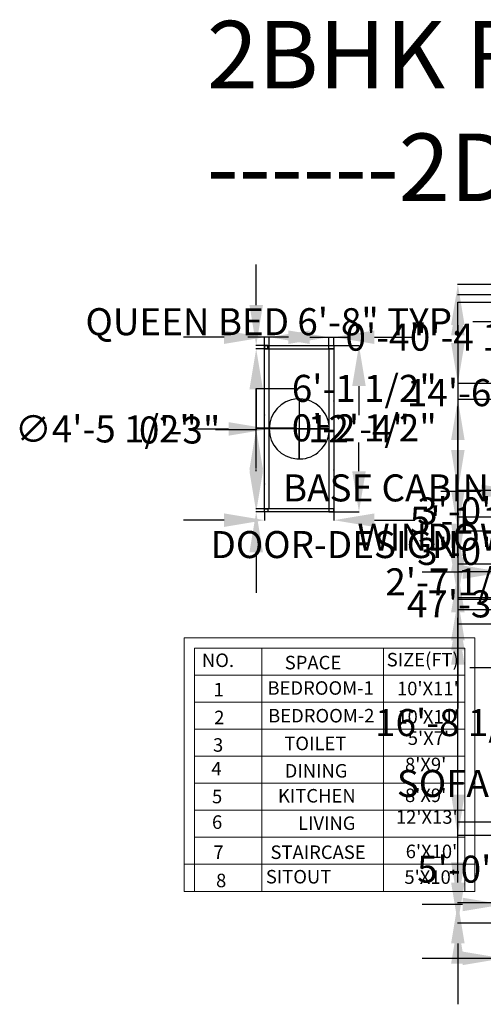
# Model space of a CAD drawing. Units: inches. Extents: x 2838 to 4029, y 1041 to 1915.
# Tile 1 of 16: x 2838 to 3250, y 1041 to 1915. Entities that reach past the tile are written whole.
import ezdxf

# ---------------------------------------------------------------- set-up
doc = ezdxf.new("R2010")
doc.units = ezdxf.units.IN
doc.header["$MEASUREMENT"] = 0
for name, color, linetype, lineweight in [('A-ANNO-DIMS', 2, 'Continuous', 18), ('A-ANNO-SCHD', 7, 'Continuous', 18), ('A-ANNO-TEXT', 7, 'Continuous', 18), ('A-DETL', 7, 'Continuous', 25), ('A-REFR', 8, 'Continuous', 13)]:
    doc.layers.add(name, color=color, linetype=linetype, lineweight=lineweight)
doc.styles.get("Standard").update_dxf_attribs({"font": 'arial.ttf'})
doc.dimstyles.get("Standard").update_dxf_attribs({"dimtxt": 24, "dimasz": 36, "dimexe": 0.18, "dimexo": 0.0625, "dimgap": 0.09, "dimtad": 0, "dimtih": 1, "dimtoh": 1, "dimdec": 0, "dimzin": 0, "dimdsep": 46, "dimlunit": 3, "dimtxsty": 'Standard', "dimcen": 0.09, "dimadec": 0, "dimazin": 0, "dimtfac": 1, "dimtdec": 0, "dimtofl": 0, "dimtmove": 0, "dimatfit": 3, "dimfxl": 1, "dimtolj": 1, "dimtzin": 0, "dimarcsym": 0})

# ---------------------------------------------------------------- blocks, each defined once
blk = doc.blocks.new('*D19')
at = {"layer": 'A-ANNO-DIMS', "color": 0, "lineweight": -2, "transparency": 16777216}
for p, q in [((3117.42, 1626.15), (3139.86, 1626.15)), ((3139.68, 1590.15), (3139.68, 1564.51)), ((3139.68, 1514.59), (3139.68, 1540.23)), ((3117.42, 1478.59), (3139.86, 1478.59))]:
    blk.add_line(p, q, dxfattribs=at)
at = {"layer": 'A-ANNO-DIMS', "color": 0, "transparency": 16777216}
for points in [[(3133.68, 1590.15), (3145.68, 1590.15), (3139.68, 1626.15)], [(3133.68, 1514.59), (3145.68, 1514.59), (3139.68, 1478.59)]]:
    blk.add_solid(points, dxfattribs=at)
at = {"layer": 'Defpoints', "color": 0, "transparency": 16777216}
for p in [(3117.35, 1626.15), (3117.35, 1478.59), (3139.68, 1478.59)]:
    blk.add_point(p, dxfattribs=at)
at = {"layer": 'A-ANNO-DIMS', "color": 0, "transparency": 16777216, "insert": (3139.68, 1552.37), "char_height": 24, "attachment_point": 5}
blk.add_mtext('\\A1;12\'-4"', dxfattribs=at)
blk = doc.blocks.new('*D25')
at = {"layer": 'A-ANNO-DIMS', "color": 0, "lineweight": -2, "transparency": 16777216}
for p, q in [((3283.93, 1516.17), (3283.93, 1552.17)), ((3276.79, 1480.17), (3284.11, 1480.17)), ((3276.79, 1432.17), (3284.11, 1432.17)), ((3283.93, 1396.17), (3283.93, 1360.17))]:
    blk.add_line(p, q, dxfattribs=at)
at = {"layer": 'A-ANNO-DIMS', "color": 0, "transparency": 16777216}
for points in [[(3277.93, 1516.17), (3289.93, 1516.17), (3283.93, 1480.17)], [(3277.93, 1396.17), (3289.93, 1396.17), (3283.93, 1432.17)]]:
    blk.add_solid(points, dxfattribs=at)
at = {"layer": 'Defpoints', "color": 0, "transparency": 16777216}
for p in [(3276.73, 1480.17), (3283.93, 1480.17), (3276.73, 1432.17)]:
    blk.add_point(p, dxfattribs=at)
at = {"layer": 'A-ANNO-DIMS', "color": 0, "transparency": 16777216, "insert": (3283.93, 1456.17), "char_height": 24, "attachment_point": 5}
blk.add_mtext('\\A1;WINDOW 4\'-0" TYP.', dxfattribs=at)
blk = doc.blocks.new('*D26')
at = {"layer": 'A-ANNO-DIMS', "color": 0, "lineweight": -2, "transparency": 16777216}
for p, q in [((3231.73, 1424.97), (3195.73, 1424.97)), ((3267.73, 1432.1), (3267.73, 1424.79)), ((3276.73, 1432.1), (3276.73, 1424.79)), ((3312.73, 1424.97), (3348.73, 1424.97))]:
    blk.add_line(p, q, dxfattribs=at)
at = {"layer": 'A-ANNO-DIMS', "color": 0, "transparency": 16777216}
for points in [[(3231.73, 1430.97), (3231.73, 1418.97), (3267.73, 1424.97)], [(3312.73, 1430.97), (3312.73, 1418.97), (3276.73, 1424.97)]]:
    blk.add_solid(points, dxfattribs=at)
at = {"layer": 'Defpoints', "color": 0, "transparency": 16777216}
for p in [(3267.73, 1432.17), (3276.73, 1432.17), (3276.73, 1424.97)]:
    blk.add_point(p, dxfattribs=at)
at = {"layer": 'A-ANNO-DIMS', "color": 0, "transparency": 16777216, "insert": (3421.97, 1424.97), "char_height": 24, "attachment_point": 5}
blk.add_mtext('\\A1;0\'-9" TYP.', dxfattribs=at)
blk = doc.blocks.new('*D29')
at = {"layer": 'A-ANNO-DIMS', "color": 0, "lineweight": -2, "transparency": 16777216}
for p, q in [((3310.15, 1348.85), (3310.15, 1339.73)), ((3370.15, 1348.85), (3370.15, 1339.73)), ((3274.15, 1339.91), (3238.15, 1339.91)), ((3406.15, 1339.91), (3442.15, 1339.91))]:
    blk.add_line(p, q, dxfattribs=at)
at = {"layer": 'A-ANNO-DIMS', "color": 0, "transparency": 16777216}
for points in [[(3274.15, 1345.91), (3274.15, 1333.91), (3310.15, 1339.91)], [(3406.15, 1345.91), (3406.15, 1333.91), (3370.15, 1339.91)]]:
    blk.add_solid(points, dxfattribs=at)
at = {"layer": 'Defpoints', "color": 0, "transparency": 16777216}
for p in [(3310.15, 1348.91), (3370.15, 1348.91), (3370.15, 1339.91)]:
    blk.add_point(p, dxfattribs=at)
at = {"layer": 'A-ANNO-DIMS', "color": 0, "transparency": 16777216, "insert": (3566.77, 1339.91), "char_height": 24, "attachment_point": 5}
blk.add_mtext('\\A1;LOVESEAT 5\'-0"', dxfattribs=at)
blk = doc.blocks.new('*D37')
at = {"layer": 'A-ANNO-DIMS', "color": 0, "lineweight": -2, "transparency": 16777216}
for p, q in [((3276.73, 1647.36), (3240.73, 1647.36)), ((3276.73, 1635.42), (3276.73, 1647.54)), ((3320.73, 1647.36), (3312.73, 1647.36)), ((3356.73, 1635.42), (3356.73, 1647.54))]:
    blk.add_line(p, q, dxfattribs=at)
at = {"layer": 'A-ANNO-DIMS', "color": 0, "transparency": 16777216}
for points in [[(3312.73, 1653.36), (3312.73, 1641.36), (3276.73, 1647.36)], [(3320.73, 1653.36), (3320.73, 1641.36), (3356.73, 1647.36)]]:
    blk.add_solid(points, dxfattribs=at)
at = {"layer": 'Defpoints', "color": 0, "transparency": 16777216}
for p in [(3276.73, 1647.36), (3276.73, 1635.36), (3356.73, 1635.36)]:
    blk.add_point(p, dxfattribs=at)
at = {"layer": 'A-ANNO-DIMS', "color": 0, "transparency": 16777216, "insert": (3064.12, 1647.36), "char_height": 24, "attachment_point": 5}
blk.add_mtext('\\A1;QUEEN BED 6\'-8" TYP.', dxfattribs=at)
blk = doc.blocks.new('*D41')
at = {"layer": 'A-ANNO-DIMS', "color": 0, "lineweight": -2, "transparency": 16777216}
for p, q in [((3284.24, 1506.2), (3284.24, 1496.56)), ((3347.73, 1506.2), (3347.73, 1496.56)), ((3248.24, 1496.74), (3212.24, 1496.74)), ((3383.73, 1496.74), (3419.73, 1496.74))]:
    blk.add_line(p, q, dxfattribs=at)
at = {"layer": 'A-ANNO-DIMS', "color": 0, "transparency": 16777216}
for points in [[(3248.24, 1502.74), (3248.24, 1490.74), (3284.24, 1496.74)], [(3383.73, 1502.74), (3383.73, 1490.74), (3347.73, 1496.74)]]:
    blk.add_solid(points, dxfattribs=at)
at = {"layer": 'Defpoints', "color": 0, "transparency": 16777216}
for p in [(3284.24, 1506.26), (3347.73, 1506.26), (3347.73, 1496.74)]:
    blk.add_point(p, dxfattribs=at)
at = {"layer": 'A-ANNO-DIMS', "color": 0, "transparency": 16777216, "insert": (3624.81, 1496.74), "char_height": 24, "attachment_point": 5}
blk.add_mtext('\\A1;WARDROBE 5\'-3 1/2" TYP.', dxfattribs=at)
blk = doc.blocks.new('*D43')
at = {"layer": 'A-ANNO-DIMS', "color": 0, "lineweight": -2, "transparency": 16777216}
for p, q in [((3231.73, 1129.95), (3195.73, 1129.95)), ((3267.73, 1131.23), (3267.73, 1129.77)), ((3276.73, 1131.23), (3276.73, 1129.77)), ((3312.73, 1129.95), (3348.73, 1129.95))]:
    blk.add_line(p, q, dxfattribs=at)
at = {"layer": 'A-ANNO-DIMS', "color": 0, "transparency": 16777216}
for points in [[(3231.73, 1135.95), (3231.73, 1123.95), (3267.73, 1129.95)], [(3312.73, 1135.95), (3312.73, 1123.95), (3276.73, 1129.95)]]:
    blk.add_solid(points, dxfattribs=at)
at = {"layer": 'Defpoints', "color": 0, "transparency": 16777216}
for p in [(3267.73, 1131.3), (3276.73, 1131.3), (3276.73, 1129.95)]:
    blk.add_point(p, dxfattribs=at)
at = {"layer": 'A-ANNO-DIMS', "color": 0, "transparency": 16777216, "insert": (3465.15, 1129.95), "char_height": 24, "attachment_point": 5}
blk.add_mtext('\\A1;PIER 0\'-9" TYP.', dxfattribs=at)
blk = doc.blocks.new('*D51')
at = {"layer": 'A-ANNO-DIMS', "color": 0, "lineweight": -2, "transparency": 16777216}
for p, q in [((3384.81, 1357.41), (3372.09, 1357.41)), ((3372.27, 1321.41), (3372.27, 1309.41)), ((3384.81, 1273.41), (3372.09, 1273.41)), ((3372.27, 1273.41), (3372.27, 1237.41)), ((3372.27, 1237.41), (3336.27, 1237.41))]:
    blk.add_line(p, q, dxfattribs=at)
at = {"layer": 'A-ANNO-DIMS', "color": 0, "transparency": 16777216}
for points in [[(3366.27, 1321.41), (3378.27, 1321.41), (3372.27, 1357.41)], [(3366.27, 1309.41), (3378.27, 1309.41), (3372.27, 1273.41)]]:
    blk.add_solid(points, dxfattribs=at)
at = {"layer": 'Defpoints', "color": 0, "transparency": 16777216}
for p in [(3384.87, 1357.41), (3372.27, 1273.41), (3384.87, 1273.41)]:
    blk.add_point(p, dxfattribs=at)
at = {"layer": 'A-ANNO-DIMS', "color": 0, "transparency": 16777216, "insert": (3254.04, 1237.41), "char_height": 24, "attachment_point": 5}
blk.add_mtext('\\A1;SOFA 7\'-0"', dxfattribs=at)
blk = doc.blocks.new('*D55')
at = {"layer": 'A-ANNO-DIMS', "color": 0, "lineweight": -2, "transparency": 16777216}
for p, q in [((3491.76, 1499.78), (3455.76, 1499.78)), ((3527.76, 1494.67), (3527.76, 1499.96)), ((3562.26, 1494.67), (3562.26, 1499.96)), ((3598.26, 1499.78), (3634.26, 1499.78))]:
    blk.add_line(p, q, dxfattribs=at)
at = {"layer": 'A-ANNO-DIMS', "color": 0, "transparency": 16777216}
for points in [[(3491.76, 1505.78), (3491.76, 1493.78), (3527.76, 1499.78)], [(3598.26, 1505.78), (3598.26, 1493.78), (3562.26, 1499.78)]]:
    blk.add_solid(points, dxfattribs=at)
at = {"layer": 'Defpoints', "color": 0, "transparency": 16777216}
for p in [(3527.76, 1499.78), (3527.76, 1494.6), (3562.26, 1494.6)]:
    blk.add_point(p, dxfattribs=at)
at = {"layer": 'A-ANNO-DIMS', "color": 0, "transparency": 16777216, "insert": (3260.33, 1499.78), "char_height": 24, "attachment_point": 5}
blk.add_mtext('\\A1;BASE CABINET 2\'-10 1/2"', dxfattribs=at)
blk = doc.blocks.new('*D59')
at = {"layer": 'A-ANNO-DIMS', "color": 0, "lineweight": -2, "transparency": 16777216}
for p, q in [((3055.85, 1478.53), (3055.85, 1470.96)), ((3117.35, 1478.53), (3117.35, 1470.96)), ((3019.85, 1471.14), (2983.85, 1471.14)), ((3153.35, 1471.14), (3189.35, 1471.14))]:
    blk.add_line(p, q, dxfattribs=at)
at = {"layer": 'A-ANNO-DIMS', "color": 0, "transparency": 16777216}
for points in [[(3019.85, 1477.14), (3019.85, 1465.14), (3055.85, 1471.14)], [(3153.35, 1477.14), (3153.35, 1465.14), (3117.35, 1471.14)]]:
    blk.add_solid(points, dxfattribs=at)
at = {"layer": 'Defpoints', "color": 0, "transparency": 16777216}
for p in [(3055.85, 1478.59), (3117.35, 1478.59), (3117.35, 1471.14)]:
    blk.add_point(p, dxfattribs=at)
at = {"layer": 'A-ANNO-DIMS', "color": 0, "transparency": 16777216, "insert": (3249.3, 1471.14), "char_height": 24, "attachment_point": 5}
blk.add_mtext('\\A1;5\'-1 1/2"', dxfattribs=at)
blk = doc.blocks.new('*D60')
at = {"layer": 'A-ANNO-DIMS', "color": 0, "lineweight": -2, "transparency": 16777216}
for p, q in [((3048.4, 1552.15), (3048.4, 1588.15)), ((3048.4, 1588.15), (3084.4, 1588.15)), ((3086.54, 1552.15), (3048.22, 1552.15)), ((3048.4, 1514.59), (3048.4, 1516.15)), ((3055.78, 1478.59), (3048.22, 1478.59))]:
    blk.add_line(p, q, dxfattribs=at)
at = {"layer": 'A-ANNO-DIMS', "color": 0, "transparency": 16777216}
for points in [[(3042.4, 1516.15), (3054.4, 1516.15), (3048.4, 1552.15)], [(3042.4, 1514.59), (3054.4, 1514.59), (3048.4, 1478.59)]]:
    blk.add_solid(points, dxfattribs=at)
at = {"layer": 'Defpoints', "color": 0, "transparency": 16777216}
for p in [(3048.4, 1552.15), (3086.6, 1552.15), (3055.85, 1478.59)]:
    blk.add_point(p, dxfattribs=at)
at = {"layer": 'A-ANNO-DIMS', "color": 0, "transparency": 16777216, "insert": (3144.41, 1588.15), "char_height": 24, "attachment_point": 5}
blk.add_mtext('\\A1;6\'-1 1/2"', dxfattribs=at)
blk = doc.blocks.new('*D61')
at = {"layer": 'A-ANNO-DIMS', "color": 0, "lineweight": -2, "transparency": 16777216}
for p, q in [((3019.85, 1633.6), (2983.85, 1633.6)), ((3055.85, 1626.21), (3055.85, 1633.78)), ((3059.9, 1623.27), (3059.9, 1633.78)), ((3095.9, 1633.6), (3131.9, 1633.6))]:
    blk.add_line(p, q, dxfattribs=at)
at = {"layer": 'A-ANNO-DIMS', "color": 0, "transparency": 16777216}
for points in [[(3019.85, 1639.6), (3019.85, 1627.6), (3055.85, 1633.6)], [(3095.9, 1639.6), (3095.9, 1627.6), (3059.9, 1633.6)]]:
    blk.add_solid(points, dxfattribs=at)
at = {"layer": 'Defpoints', "color": 0, "transparency": 16777216}
for p in [(3055.85, 1626.15), (3059.9, 1633.6), (3059.9, 1623.2)]:
    blk.add_point(p, dxfattribs=at)
at = {"layer": 'A-ANNO-DIMS', "color": 0, "transparency": 16777216, "insert": (3163.89, 1633.6), "char_height": 24, "attachment_point": 5}
blk.add_mtext('\\A1;0\'-4"', dxfattribs=at)
blk = doc.blocks.new('*D62')
at = {"layer": 'A-ANNO-DIMS', "color": 0, "lineweight": -2, "transparency": 16777216}
for p, q in [((3048.4, 1662.15), (3048.4, 1698.15)), ((3055.78, 1626.15), (3048.22, 1626.15)), ((3059.84, 1623.2), (3048.22, 1623.2)), ((3048.4, 1587.2), (3048.4, 1551.2)), ((3048.4, 1551.2), (3012.4, 1551.2))]:
    blk.add_line(p, q, dxfattribs=at)
at = {"layer": 'A-ANNO-DIMS', "color": 0, "transparency": 16777216}
for points in [[(3042.4, 1662.15), (3054.4, 1662.15), (3048.4, 1626.15)], [(3042.4, 1587.2), (3054.4, 1587.2), (3048.4, 1623.2)]]:
    blk.add_solid(points, dxfattribs=at)
at = {"layer": 'Defpoints', "color": 0, "transparency": 16777216}
for p in [(3055.85, 1626.15), (3048.4, 1623.2), (3059.9, 1623.2)]:
    blk.add_point(p, dxfattribs=at)
at = {"layer": 'A-ANNO-DIMS', "color": 0, "transparency": 16777216, "insert": (2980.41, 1551.2), "char_height": 24, "attachment_point": 5}
blk.add_mtext('\\A1;0\'-3"', dxfattribs=at)
blk = doc.blocks.new('*D63')
at = {"layer": 'A-ANNO-DIMS', "color": 0, "lineweight": -2, "transparency": 16777216}
for p, q in [((3048.4, 1517.1), (3048.4, 1553.1)), ((3048.4, 1553.1), (3084.4, 1553.1)), ((3059.84, 1481.1), (3048.22, 1481.1)), ((3055.78, 1478.59), (3048.22, 1478.59)), ((3048.4, 1442.59), (3048.4, 1406.59))]:
    blk.add_line(p, q, dxfattribs=at)
at = {"layer": 'A-ANNO-DIMS', "color": 0, "transparency": 16777216}
for points in [[(3042.4, 1517.1), (3054.4, 1517.1), (3048.4, 1481.1)], [(3042.4, 1442.59), (3054.4, 1442.59), (3048.4, 1478.59)]]:
    blk.add_solid(points, dxfattribs=at)
at = {"layer": 'Defpoints', "color": 0, "transparency": 16777216}
for p in [(3048.4, 1481.1), (3055.85, 1478.59), (3059.9, 1481.1)]:
    blk.add_point(p, dxfattribs=at)
at = {"layer": 'A-ANNO-DIMS', "color": 0, "transparency": 16777216, "insert": (3144.35, 1553.1), "char_height": 24, "attachment_point": 5}
blk.add_mtext('\\A1;0\'-2 1/2"', dxfattribs=at)
blk = doc.blocks.new('*D64')
at = {"layer": 'A-ANNO-DIMS', "color": 0, "lineweight": -2, "transparency": 16777216}
for p, q in [((3076.99, 1633.6), (3040.99, 1633.6)), ((3112.99, 1623.27), (3112.99, 1633.78)), ((3117.35, 1626.21), (3117.35, 1633.78)), ((3153.35, 1633.6), (3189.35, 1633.6))]:
    blk.add_line(p, q, dxfattribs=at)
at = {"layer": 'A-ANNO-DIMS', "color": 0, "transparency": 16777216}
for points in [[(3076.99, 1639.6), (3076.99, 1627.6), (3112.99, 1633.6)], [(3153.35, 1639.6), (3153.35, 1627.6), (3117.35, 1633.6)]]:
    blk.add_solid(points, dxfattribs=at)
at = {"layer": 'Defpoints', "color": 0, "transparency": 16777216}
for p in [(3117.35, 1633.6), (3117.35, 1626.15), (3112.99, 1623.2)]:
    blk.add_point(p, dxfattribs=at)
at = {"layer": 'A-ANNO-DIMS', "color": 0, "transparency": 16777216, "insert": (3249.3, 1633.6), "char_height": 24, "attachment_point": 5}
blk.add_mtext('\\A1;0\'-4 1/2"', dxfattribs=at)
blk = doc.blocks.new('*D66')
at = {"layer": 'A-ANNO-DIMS', "color": 0, "lineweight": -2, "transparency": 16777216}
for p, q in [((3227.506626, 1227.297346), (3227.506626, 1263.297346)), ((3267.669126, 1191.297346), (3227.326626, 1191.297346)), ((3267.669126, 1131.297346), (3227.326626, 1131.297346)), ((3227.506626, 1095.297346), (3227.506626, 1059.297346))]:
    blk.add_line(p, q, dxfattribs=at)
at = {"layer": 'A-ANNO-DIMS', "color": 0, "transparency": 16777216}
for points in [[(3221.506626, 1227.297346), (3233.506626, 1227.297346), (3227.506626, 1191.297346)], [(3221.506626, 1095.297346), (3233.506626, 1095.297346), (3227.506626, 1131.297346)]]:
    blk.add_solid(points, dxfattribs=at)
at = {"layer": 'Defpoints', "color": 0, "transparency": 16777216}
for p in [(3267.731626, 1191.297346), (3227.506626, 1131.297346), (3267.731626, 1131.297346)]:
    blk.add_point(p, dxfattribs=at)
at = {"layer": 'A-ANNO-DIMS', "color": 0, "transparency": 16777216, "insert": (3227.506626, 1161.297346), "char_height": 24, "attachment_point": 5}
blk.add_mtext('\\A1;5\'-0"', dxfattribs=at)
blk = doc.blocks.new('*D67')
at = {"layer": 'A-ANNO-DIMS', "color": 0, "lineweight": -2, "transparency": 16777216}
for p, q in [((3258.67, 1680.3), (3227.33, 1680.3)), ((3227.51, 1644.3), (3227.51, 1409.15)), ((3227.51, 1149.3), (3227.51, 1384.45)), ((3329.6, 1113.3), (3227.33, 1113.3))]:
    blk.add_line(p, q, dxfattribs=at)
at = {"layer": 'A-ANNO-DIMS', "color": 0, "transparency": 16777216}
for points in [[(3221.51, 1644.3), (3233.51, 1644.3), (3227.51, 1680.3)], [(3221.51, 1149.3), (3233.51, 1149.3), (3227.51, 1113.3)]]:
    blk.add_solid(points, dxfattribs=at)
at = {"layer": 'Defpoints', "color": 0, "transparency": 16777216}
for p in [(3227.51, 1680.3), (3258.73, 1680.3), (3329.66, 1113.3)]:
    blk.add_point(p, dxfattribs=at)
at = {"layer": 'A-ANNO-DIMS', "color": 0, "transparency": 16777216, "insert": (3227.51, 1396.8), "char_height": 24, "attachment_point": 5}
blk.add_mtext('\\A1;47\'-3"', dxfattribs=at)
blk = doc.blocks.new('*D69')
at = {"layer": 'A-ANNO-DIMS', "color": 0, "lineweight": -2, "transparency": 16777216}
for p, q in [((3300.731626, 1191.234846), (3300.731626, 1081.892346)), ((3372.731626, 1191.234846), (3372.731626, 1081.892346)), ((3264.731626, 1082.072346), (3228.731626, 1082.072346)), ((3408.731626, 1082.072346), (3444.731626, 1082.072346))]:
    blk.add_line(p, q, dxfattribs=at)
at = {"layer": 'A-ANNO-DIMS', "color": 0, "transparency": 16777216}
for points in [[(3264.731626, 1088.072346), (3264.731626, 1076.072346), (3300.731626, 1082.072346)], [(3408.731626, 1088.072346), (3408.731626, 1076.072346), (3372.731626, 1082.072346)]]:
    blk.add_solid(points, dxfattribs=at)
at = {"layer": 'Defpoints', "color": 0, "transparency": 16777216}
for p in [(3300.731626, 1191.297346), (3372.731626, 1191.297346), (3372.731626, 1082.072346)]:
    blk.add_point(p, dxfattribs=at)
at = {"layer": 'A-ANNO-DIMS', "color": 0, "transparency": 16777216, "insert": (3336.731626, 1082.072346), "char_height": 24, "attachment_point": 5}
blk.add_mtext('\\A1;6\'-0"', dxfattribs=at)
blk = doc.blocks.new('*D71')
at = {"layer": 'A-ANNO-DIMS', "color": 0, "lineweight": -2, "transparency": 16777216}
for p, q in [((3267.73, 1131.23), (3267.73, 1081.89)), ((3329.66, 1113.23), (3329.66, 1081.89)), ((3231.73, 1082.07), (3195.73, 1082.07)), ((3365.66, 1082.07), (3401.66, 1082.07))]:
    blk.add_line(p, q, dxfattribs=at)
at = {"layer": 'A-ANNO-DIMS', "color": 0, "transparency": 16777216}
for points in [[(3231.73, 1088.07), (3231.73, 1076.07), (3267.73, 1082.07)], [(3365.66, 1088.07), (3365.66, 1076.07), (3329.66, 1082.07)]]:
    blk.add_solid(points, dxfattribs=at)
at = {"layer": 'Defpoints', "color": 0, "transparency": 16777216}
for p in [(3267.73, 1131.3), (3329.66, 1113.3), (3329.66, 1082.07)]:
    blk.add_point(p, dxfattribs=at)
at = {"layer": 'A-ANNO-DIMS', "color": 0, "transparency": 16777216, "insert": (3433.65, 1082.07), "char_height": 24, "attachment_point": 5}
blk.add_mtext('\\A1;5\'-2"', dxfattribs=at)
blk = doc.blocks.new('*D72')
at = {"layer": 'A-ANNO-DIMS', "color": 0, "lineweight": -2, "transparency": 16777216}
for p, q in [((3227.51, 1167.3), (3227.51, 1203.3)), ((3227.51, 1203.3), (3263.51, 1203.3)), ((3329.6, 1131.3), (3227.33, 1131.3)), ((3329.6, 1113.3), (3227.33, 1113.3)), ((3227.51, 1077.3), (3227.51, 1041.3))]:
    blk.add_line(p, q, dxfattribs=at)
at = {"layer": 'A-ANNO-DIMS', "color": 0, "transparency": 16777216}
for points in [[(3221.51, 1167.3), (3233.51, 1167.3), (3227.51, 1131.3)], [(3221.51, 1077.3), (3233.51, 1077.3), (3227.51, 1113.3)]]:
    blk.add_solid(points, dxfattribs=at)
at = {"layer": 'Defpoints', "color": 0, "transparency": 16777216}
for p in [(3227.51, 1131.3), (3329.66, 1131.3), (3329.66, 1113.3)]:
    blk.add_point(p, dxfattribs=at)
at = {"layer": 'A-ANNO-DIMS', "color": 0, "transparency": 16777216, "insert": (3294.37, 1203.3), "char_height": 24, "attachment_point": 5}
blk.add_mtext('\\A1;1\'-6"', dxfattribs=at)
blk = doc.blocks.new('*D76')
at = {"layer": 'A-ANNO-DIMS', "color": 0, "lineweight": -2, "transparency": 16777216}
for p, q in [((3276.67, 1391.57), (3227.33, 1391.57)), ((3227.51, 1355.57), (3227.51, 1303.94)), ((3227.51, 1227.3), (3227.51, 1278.94)), ((3267.67, 1191.3), (3227.33, 1191.3))]:
    blk.add_line(p, q, dxfattribs=at)
at = {"layer": 'A-ANNO-DIMS', "color": 0, "transparency": 16777216}
for points in [[(3221.51, 1355.57), (3233.51, 1355.57), (3227.51, 1391.57)], [(3221.51, 1227.3), (3233.51, 1227.3), (3227.51, 1191.3)]]:
    blk.add_solid(points, dxfattribs=at)
at = {"layer": 'Defpoints', "color": 0, "transparency": 16777216}
for p in [(3227.51, 1391.57), (3276.73, 1391.57), (3267.73, 1191.3)]:
    blk.add_point(p, dxfattribs=at)
at = {"layer": 'A-ANNO-DIMS', "color": 0, "transparency": 16777216, "insert": (3227.51, 1291.44), "char_height": 24, "attachment_point": 5}
blk.add_mtext('\\A1;16\'-8 1/2"', dxfattribs=at)
blk = doc.blocks.new('*D77')
at = {"layer": 'A-ANNO-DIMS', "color": 0, "lineweight": -2, "transparency": 16777216}
for p, q in [((3267.67, 1671.3), (3227.33, 1671.3)), ((3227.51, 1635.3), (3227.51, 1596.69)), ((3227.51, 1533.39), (3227.51, 1572)), ((3276.67, 1497.39), (3227.33, 1497.39))]:
    blk.add_line(p, q, dxfattribs=at)
at = {"layer": 'A-ANNO-DIMS', "color": 0, "transparency": 16777216}
for points in [[(3221.51, 1635.3), (3233.51, 1635.3), (3227.51, 1671.3)], [(3221.51, 1533.39), (3233.51, 1533.39), (3227.51, 1497.39)]]:
    blk.add_solid(points, dxfattribs=at)
at = {"layer": 'Defpoints', "color": 0, "transparency": 16777216}
for p in [(3227.51, 1671.3), (3267.73, 1671.3), (3276.73, 1497.39)]:
    blk.add_point(p, dxfattribs=at)
at = {"layer": 'A-ANNO-DIMS', "color": 0, "transparency": 16777216, "insert": (3227.51, 1584.35), "char_height": 24, "attachment_point": 5}
blk.add_mtext('\\A1;14\'-6"', dxfattribs=at)
blk = doc.blocks.new('*D81')
at = {"layer": 'A-ANNO-DIMS', "color": 0, "lineweight": -2, "transparency": 16777216}
for p, q in [((3267.73, 1191.23), (3267.73, 1081.89)), ((3300.73, 1191.23), (3300.73, 1081.89)), ((3231.73, 1082.07), (3195.73, 1082.07)), ((3336.73, 1082.07), (3372.73, 1082.07))]:
    blk.add_line(p, q, dxfattribs=at)
at = {"layer": 'A-ANNO-DIMS', "color": 0, "transparency": 16777216}
for points in [[(3231.73, 1088.07), (3231.73, 1076.07), (3267.73, 1082.07)], [(3336.73, 1088.07), (3336.73, 1076.07), (3300.73, 1082.07)]]:
    blk.add_solid(points, dxfattribs=at)
at = {"layer": 'Defpoints', "color": 0, "transparency": 16777216}
for p in [(3267.73, 1191.3), (3300.73, 1191.3), (3300.73, 1082.07)]:
    blk.add_point(p, dxfattribs=at)
at = {"layer": 'A-ANNO-DIMS', "color": 0, "transparency": 16777216, "insert": (3404.93, 1082.07), "char_height": 24, "attachment_point": 5}
blk.add_mtext('\\A1;2\'-9"', dxfattribs=at)
blk = doc.blocks.new('*D87')
at = {"layer": 'A-ANNO-DIMS', "color": 0, "lineweight": -2, "transparency": 16777216}
for p, q in [((3227.506626, 1497.394218), (3227.506626, 1533.394218)), ((3513.669126, 1461.394218), (3227.326626, 1461.394218)), ((3513.669126, 1425.394218), (3227.326626, 1425.394218)), ((3227.506626, 1389.394218), (3227.506626, 1353.394218))]:
    blk.add_line(p, q, dxfattribs=at)
at = {"layer": 'A-ANNO-DIMS', "color": 0, "transparency": 16777216}
for points in [[(3221.506626, 1497.394218), (3233.506626, 1497.394218), (3227.506626, 1461.394218)], [(3221.506626, 1389.394218), (3233.506626, 1389.394218), (3227.506626, 1425.394218)]]:
    blk.add_solid(points, dxfattribs=at)
at = {"layer": 'Defpoints', "color": 0, "transparency": 16777216}
for p in [(3227.506626, 1461.394218), (3513.731626, 1461.394218), (3513.731626, 1425.394218)]:
    blk.add_point(p, dxfattribs=at)
at = {"layer": 'A-ANNO-DIMS', "color": 0, "transparency": 16777216, "insert": (3227.506626, 1443.394218), "char_height": 24, "attachment_point": 5}
blk.add_mtext('\\A1;3\'-0"', dxfattribs=at)
blk = doc.blocks.new('*D91')
at = {"layer": 'A-ANNO-DIMS', "color": 0, "lineweight": -2, "transparency": 16777216}
for p, q in [((3227.506626, 1533.394218), (3227.506626, 1569.394218)), ((3522.669126, 1497.394218), (3227.326626, 1497.394218)), ((3522.669126, 1461.394218), (3227.326626, 1461.394218)), ((3227.506626, 1425.394218), (3227.506626, 1389.394218))]:
    blk.add_line(p, q, dxfattribs=at)
at = {"layer": 'A-ANNO-DIMS', "color": 0, "transparency": 16777216}
for points in [[(3221.506626, 1533.394218), (3233.506626, 1533.394218), (3227.506626, 1497.394218)], [(3221.506626, 1425.394218), (3233.506626, 1425.394218), (3227.506626, 1461.394218)]]:
    blk.add_solid(points, dxfattribs=at)
at = {"layer": 'Defpoints', "color": 0, "transparency": 16777216}
for p in [(3522.731626, 1497.394218), (3227.506626, 1461.394218), (3522.731626, 1461.394218)]:
    blk.add_point(p, dxfattribs=at)
at = {"layer": 'A-ANNO-DIMS', "color": 0, "transparency": 16777216, "insert": (3227.506626, 1479.394218), "char_height": 24, "attachment_point": 5}
blk.add_mtext('\\A1;3\'-0"', dxfattribs=at)
blk = doc.blocks.new('*D93')
at = {"layer": 'A-ANNO-DIMS', "color": 0, "lineweight": -2, "transparency": 16777216}
for p, q in [((3227.51, 1438.06), (3227.51, 1474.06)), ((3227.51, 1474.06), (3263.51, 1474.06)), ((3522.67, 1402.06), (3227.33, 1402.06)), ((3522.67, 1378.73), (3227.33, 1378.73)), ((3227.51, 1342.73), (3227.51, 1306.73))]:
    blk.add_line(p, q, dxfattribs=at)
at = {"layer": 'A-ANNO-DIMS', "color": 0, "transparency": 16777216}
for points in [[(3221.51, 1438.06), (3233.51, 1438.06), (3227.51, 1402.06)], [(3221.51, 1342.73), (3233.51, 1342.73), (3227.51, 1378.73)]]:
    blk.add_solid(points, dxfattribs=at)
at = {"layer": 'Defpoints', "color": 0, "transparency": 16777216}
for p in [(3227.51, 1402.06), (3522.73, 1402.06), (3522.73, 1378.73)]:
    blk.add_point(p, dxfattribs=at)
at = {"layer": 'A-ANNO-DIMS', "color": 0, "transparency": 16777216, "insert": (3331.65, 1474.06), "char_height": 24, "attachment_point": 5}
blk.add_mtext('\\A1;1\'-11 1/2"', dxfattribs=at)
blk = doc.blocks.new('*D95')
at = {"layer": 'A-ANNO-DIMS', "color": 0, "lineweight": -2, "transparency": 16777216}
for p, q in [((3227.51, 1468.17), (3227.51, 1504.17)), ((3276.67, 1432.17), (3227.33, 1432.17)), ((3276.67, 1400.57), (3227.33, 1400.57)), ((3227.51, 1364.57), (3227.51, 1328.57))]:
    blk.add_line(p, q, dxfattribs=at)
at = {"layer": 'A-ANNO-DIMS', "color": 0, "transparency": 16777216}
for points in [[(3221.51, 1468.17), (3233.51, 1468.17), (3227.51, 1432.17)], [(3221.51, 1364.57), (3233.51, 1364.57), (3227.51, 1400.57)]]:
    blk.add_solid(points, dxfattribs=at)
at = {"layer": 'Defpoints', "color": 0, "transparency": 16777216}
for p in [(3227.51, 1432.17), (3276.73, 1432.17), (3276.73, 1400.57)]:
    blk.add_point(p, dxfattribs=at)
at = {"layer": 'A-ANNO-DIMS', "color": 0, "transparency": 16777216, "insert": (3227.51, 1416.37), "char_height": 24, "attachment_point": 5}
blk.add_mtext('\\A1;2\'-7 1/2"', dxfattribs=at)
blk = doc.blocks.new('*D103')
at = {"layer": 'A-ANNO-DIMS', "color": 0, "lineweight": -2, "transparency": 16777216}
for p, q in [((3227.51, 1628.55), (3227.51, 1664.55)), ((3227.51, 1664.55), (3263.51, 1664.55)), ((3469.64, 1592.55), (3227.33, 1592.55)), ((3441.67, 1578.3), (3227.33, 1578.3)), ((3227.51, 1542.3), (3227.51, 1506.3))]:
    blk.add_line(p, q, dxfattribs=at)
at = {"layer": 'A-ANNO-DIMS', "color": 0, "transparency": 16777216}
for points in [[(3221.51, 1628.55), (3233.51, 1628.55), (3227.51, 1592.55)], [(3221.51, 1542.3), (3233.51, 1542.3), (3227.51, 1578.3)]]:
    blk.add_solid(points, dxfattribs=at)
at = {"layer": 'Defpoints', "color": 0, "transparency": 16777216}
for p in [(3227.51, 1592.55), (3469.7, 1592.55), (3441.73, 1578.3)]:
    blk.add_point(p, dxfattribs=at)
at = {"layer": 'A-ANNO-DIMS', "color": 0, "transparency": 16777216, "insert": (3322.33, 1664.55), "char_height": 24, "attachment_point": 5}
blk.add_mtext('\\A1;1\'-2 1/2"', dxfattribs=at)
blk = doc.blocks.new('*D108')
at = {"layer": 'A-ANNO-DIMS', "color": 0, "lineweight": -2, "transparency": 16777216}
for p, q in [((2987.9, 1552.15), (3023.9, 1552.15)), ((3086.51, 1552.15), (3086.69, 1552.15)), ((3086.6, 1552.06), (3086.6, 1552.24))]:
    blk.add_line(p, q, dxfattribs=at)
at = {"layer": 'A-ANNO-DIMS', "color": 0, "transparency": 16777216}
blk.add_solid([(3023.9, 1558.15), (3023.9, 1546.15), (3059.9, 1552.15)], dxfattribs=at)
at = {"layer": 'Defpoints', "color": 0, "transparency": 16777216}
for p in [(3059.9, 1552.15), (3113.29, 1552.15)]:
    blk.add_point(p, dxfattribs=at)
at = {"layer": 'A-ANNO-DIMS', "color": 0, "transparency": 16777216, "insert": (2914.9, 1552.15), "char_height": 24, "attachment_point": 5}
blk.add_mtext('\\A1;∅4\'-5 1/2"', dxfattribs=at)

msp = doc.modelspace()

# ---------------------------------------------------------------- linework, layer by layer
at = {"layer": 'A-ANNO-SCHD'}
for p, q in [((3242.56, 1366.58), (2984.56, 1366.58)), ((2984.56, 1366.58), (2984.56, 1141.58)), ((3242.56, 1141.58), (3242.56, 1366.58)), ((2993.56, 1357.58), (2993.56, 1141.58)), ((3233.56, 1357.58), (2993.56, 1357.58)), ((3053.56, 1141.58), (3053.56, 1357.58)), ((3161.56, 1141.58), (3161.56, 1357.58)), ((3233.56, 1141.58), (3233.56, 1357.58)), ((3233.56, 1333.58), (2993.56, 1333.58)), ((3233.56, 1309.58), (2993.56, 1309.58)), ((3233.56, 1285.58), (2993.56, 1285.58)), ((3233.56, 1261.58), (2993.56, 1261.58)), ((3233.56, 1237.58), (2993.56, 1237.58)), ((3233.56, 1213.58), (2993.56, 1213.58)), ((3233.56, 1189.58), (2993.56, 1189.58)), ((3242.56, 1165.58), (2984.56, 1165.58)), ((3242.56, 1141.58), (2984.56, 1141.58))]:
    msp.add_line(p, q, dxfattribs=at)
at = {"layer": 'A-DETL'}
for p, q in [((3059.9, 1481.1), (3059.9, 1623.2)), ((3112.99, 1623.2), (3112.99, 1593.64)), ((3112.99, 1593.64), (3112.99, 1481.1)), ((3086.6, 1578.85), (3086.6, 1525.46)), ((3086.6, 1552.15), (3059.9, 1552.15)), ((3086.6, 1525.46), (3086.6, 1552.15)), ((3086.6, 1552.15), (3112.99, 1552.15)), ((3112.99, 1552.15), (3086.6, 1552.15)), ((3112.99, 1481.1), (3058.62, 1481.1))]:
    msp.add_line(p, q, dxfattribs=at)
for points in [[(3117.35, 1626.15), (3117.35, 1478.59), (3055.85, 1478.59), (3055.85, 1626.15)], [(3055.85, 1626.15), (3055.85, 1623.2), (3058.62, 1623.2), (3058.62, 1626.15)], [(3112.99, 1623.2), (3112.99, 1626.15), (3117.35, 1626.15), (3117.35, 1623.2)], [(3112.12, 1554.79), (3104.88, 1554.79), (3104.88, 1553.91), (3112.12, 1553.91)], [(3058.62, 1481.1), (3058.62, 1478.59), (3055.85, 1478.59), (3055.85, 1481.1)], [(3117.35, 1478.59), (3117.35, 1481.1), (3112.99, 1481.1), (3112.99, 1478.59)]]:
    msp.add_lwpolyline(points, close=True, dxfattribs=at)
for points in [[(3055.85, 1623.2), (3117.35, 1623.2)], [(3117.35, 1481.1), (3055.85, 1481.1)]]:
    msp.add_lwpolyline(points, dxfattribs=at)
msp.add_arc((3086.6, 1552.15), 26.7, 8.67275, 351.32725, dxfattribs=at)
at = {"layer": 'A-REFR'}
for p in [(3055.85, 1626.15), (3117.35, 1577.06), (3055.85, 1564.64), (3117.35, 1515.56), (3055.85, 1503.13), (3092.81, 1478.59)]:
    msp.add_point(p, dxfattribs=at)

# ---------------------------------------------------------------- texts
at = {"layer": 'A-ANNO-TEXT', "attachment_point": 1}
for s, width, insert, char_height in [('2BHK RESIDENTIAL HOUSE \\P------2D FLOOR PLAN------', 1981.8988, (3004.58, 1914.43), 60), ('DOOR-DESIGN', 85.938, (3007.84, 1461.48), 24), ('NO.', 45.9311, (3000.2, 1352.75), 12), ('SPACE', 45.9311, (3073.75, 1350.7), 12), ('SIZE(FT)', 45.9311, (3164.33, 1353.29), 12), ('1', 45.9311, (3010.52, 1326.69), 12), ('BEDROOM-1', 45.9311, (3058.41, 1328.13), 12), ("10'X11'", 45.9311, (3173.43, 1327.7), 12), ('BEDROOM-2', 45.9311, (3059, 1303.55), 12), ("10'X11'", 45.9311, (3173.74, 1302.61), 12), ('2', 45.9311, (3011.1, 1301.99), 12), ('3', 45.9311, (3010.07, 1277.55), 12), ('TOILET', 45.9311, (3073.36, 1278.93), 12), ("5'X7'", 45.9311, (3183.06, 1283.61), 12), ("8'X9'", 45.9311, (3180.56, 1260.26), 12), ('4', 45.9311, (3008.61, 1256.5), 12), ('DINING', 45.9311, (3073.67, 1254.6), 12), ('KITCHEN', 45.9311, (3067.74, 1232.45), 12), ("8'X9'", 45.9311, (3180.56, 1232.86), 12), ('5', 45.9311, (3009.16, 1231.77), 12), ('6', 45.9311, (3009.16, 1209.06), 12), ('LIVING ', 45.9311, (3085.53, 1208.12), 12), ("12'X13'", 45.9311, (3172.49, 1213.58), 12), ('7', 45.9311, (3010.41, 1182.3), 12), ('STAIRCASE', 45.9311, (3061.11, 1182.33), 12), ("6'X10'", 45.9311, (3181.19, 1183.05), 12), ('8', 45.9311, (3012.76, 1157.23), 12), ('SITOUT', 45.9311, (3057, 1160.59), 12), ("5'X10'", 45.9311, (3180.02, 1160.23), 12)]:
    msp.add_mtext_dynamic_manual_height_columns(s, width=width, gutter_width=1, heights=[0], dxfattribs=dict(at, insert=insert, char_height=char_height))

# ---------------------------------------------------------------- dimensions: what is measured, and where the dimension line sits
at = {"layer": 'A-ANNO-DIMS'}
for base, p1, p2, angle, text, picture, middle in [((3276.73, 1647.36), (3356.73, 1635.36), (3276.73, 1635.36), 180, 'QUEEN BED <> TYP.', '*D37', (3064.12, 1647.36)), ((3527.76, 1499.78), (3562.26, 1494.6), (3527.76, 1494.6), 180, 'BASE CABINET <>', '*D55', (3260.33, 1499.78)), ((3283.93, 1480.17), (3276.73, 1432.17), (3276.73, 1480.17), 90, 'WINDOW <> TYP.', '*D25', (3283.93, 1456.17)), ((3372.27, 1273.41), (3384.87, 1357.41), (3384.87, 1273.41), 270, 'SOFA <>', '*D51', (3254.04, 1237.41))]:
    dim = msp.add_linear_dim(base=base, p1=p1, p2=p2, angle=angle, text=text, dimstyle='Standard', override={"dimdec": 1, "dimlfac": 1, "dimrnd": 0, "dimzin": 1, "dimdsep": 46, "dimlunit": 4, "dimfrac": 2}, dxfattribs=at)
    dim.commit()
    dim.dimension.update_dxf_attribs({"geometry": picture, "text_midpoint": middle})
for base, p1, p2, override, picture, middle in [((3048.3954, 1623.2048), (3055.8454, 1626.1478), (3059.904, 1623.2048), {"dimdec": 1, "dimlfac": 1, "dimrnd": 0, "dimzin": 1, "dimdsep": 46, "dimlunit": 4, "dimfrac": 2}, '*D62', (2980.4064, 1551.2048)), ((3227.5066, 1592.5486), (3441.7316, 1578.2973), (3469.6999, 1592.5486), {"dimdec": 1, "dimlfac": 1, "dimrnd": 0, "dimzin": 1, "dimdsep": 46, "dimlunit": 4, "dimfrac": 2}, '*D103', (3322.3279, 1664.5486)), ((3227.51, 1680.3), (3329.66, 1113.3), (3258.73, 1680.3), {"dimdec": 1, "dimlfac": 1, "dimrnd": 0, "dimzin": 1, "dimdsep": 46, "dimlunit": 4, "dimfrac": 2}, '*D67', (3227.51, 1396.8)), ((3227.51, 1671.3), (3276.73, 1497.39), (3267.73, 1671.3), {"dimdec": 1, "dimlfac": 1, "dimrnd": 0, "dimzin": 1, "dimdsep": 46, "dimlunit": 4, "dimfrac": 2}, '*D77', (3227.51, 1584.35)), ((3139.68, 1478.59), (3117.35, 1626.15), (3117.35, 1478.59), {"dimclrd": 0, "dimclre": 0, "dimclrt": 0}, '*D19', (3139.68, 1552.37)), ((3048.4, 1552.15), (3055.85, 1478.59), (3086.6, 1552.15), {"dimdec": 1, "dimlfac": 1, "dimrnd": 0, "dimzin": 1, "dimdsep": 46, "dimlunit": 4, "dimfrac": 2}, '*D60', (3144.41, 1588.15)), ((3048.4, 1481.1), (3055.85, 1478.59), (3059.9, 1481.1), {"dimdec": 1, "dimlfac": 1, "dimrnd": 0, "dimzin": 1, "dimdsep": 46, "dimlunit": 4, "dimfrac": 2}, '*D63', (3144.35, 1553.1)), ((3227.51, 1461.39), (3522.73, 1497.39), (3522.73, 1461.39), {"dimdec": 1, "dimlfac": 1, "dimrnd": 0, "dimzin": 1, "dimdsep": 46, "dimlunit": 4, "dimfrac": 2}, '*D91', (3227.51, 1479.39)), ((3227.51, 1461.39), (3513.73, 1425.39), (3513.73, 1461.39), {"dimdec": 1, "dimlfac": 1, "dimrnd": 0, "dimzin": 1, "dimdsep": 46, "dimlunit": 4, "dimfrac": 2}, '*D87', (3227.51, 1443.39)), ((3227.51, 1432.17), (3276.73, 1400.57), (3276.73, 1432.17), {"dimdec": 1, "dimlfac": 1, "dimrnd": 0, "dimzin": 1, "dimdsep": 46, "dimlunit": 4, "dimfrac": 2}, '*D95', (3227.51, 1416.37)), ((3227.51, 1402.06), (3522.73, 1378.73), (3522.73, 1402.06), {"dimdec": 1, "dimlfac": 1, "dimrnd": 0, "dimzin": 1, "dimdsep": 46, "dimlunit": 4, "dimfrac": 2}, '*D93', (3331.65, 1474.06)), ((3227.51, 1391.57), (3267.73, 1191.3), (3276.73, 1391.57), {"dimdec": 1, "dimlfac": 1, "dimrnd": 0, "dimzin": 1, "dimdsep": 46, "dimlunit": 4, "dimfrac": 2}, '*D76', (3227.51, 1291.44)), ((3227.51, 1131.3), (3267.73, 1191.3), (3267.73, 1131.3), {"dimdec": 1, "dimlfac": 1, "dimrnd": 0, "dimzin": 1, "dimdsep": 46, "dimlunit": 4, "dimfrac": 2}, '*D66', (3227.51, 1161.3)), ((3227.51, 1131.3), (3329.66, 1113.3), (3329.66, 1131.3), {"dimdec": 1, "dimlfac": 1, "dimrnd": 0, "dimzin": 1, "dimdsep": 46, "dimlunit": 4, "dimfrac": 2}, '*D72', (3294.37, 1203.3))]:
    dim = msp.add_linear_dim(base=base, p1=p1, p2=p2, angle=90, dimstyle='Standard', override=override, dxfattribs=at)
    dim.commit()
    dim.dimension.update_dxf_attribs({"geometry": picture, "text_midpoint": middle})
for base, p1, p2, picture, middle in [((3117.35, 1633.6), (3112.99, 1623.2), (3117.35, 1626.15), '*D64', (3249.3, 1633.6)), ((3059.904, 1633.5978), (3055.8454, 1626.1478), (3059.904, 1623.2048), '*D61', (3163.8931, 1633.5978)), ((3117.35, 1471.14), (3055.85, 1478.59), (3117.35, 1478.59), '*D59', (3249.3, 1471.14)), ((3300.73, 1082.07), (3267.73, 1191.3), (3300.73, 1191.3), '*D81', (3404.93, 1082.07)), ((3372.73, 1082.07), (3300.73, 1191.3), (3372.73, 1191.3), '*D69', (3336.73, 1082.07)), ((3329.66, 1082.07), (3267.73, 1131.3), (3329.66, 1113.3), '*D71', (3433.65, 1082.07))]:
    dim = msp.add_linear_dim(base=base, p1=p1, p2=p2, dimstyle='Standard', override={"dimdec": 1, "dimlfac": 1, "dimrnd": 0, "dimzin": 1, "dimdsep": 46, "dimlunit": 4, "dimfrac": 2}, dxfattribs=at)
    dim.commit()
    dim.dimension.update_dxf_attribs({"geometry": picture, "text_midpoint": middle})
dim = msp.add_diameter_dim_2p(p1=(3113.29, 1552.15), p2=(3059.9, 1552.15), dimstyle='Standard', override={"dimdec": 1, "dimlfac": 1, "dimrnd": 0, "dimzin": 1, "dimdsep": 46, "dimlunit": 4, "dimfrac": 2}, dxfattribs=at)
dim.commit()
dim.dimension.update_dxf_attribs({"geometry": '*D108', "text_midpoint": (2987.9, 1552.15), "dimtype": 163})
for base, p1, p2, text, picture, middle in [((3347.73, 1496.74), (3284.24, 1506.26), (3347.73, 1506.26), 'WARDROBE <> TYP.', '*D41', (3624.81, 1496.74)), ((3276.73, 1424.97), (3267.73, 1432.17), (3276.73, 1432.17), '<> TYP.', '*D26', (3421.97, 1424.97)), ((3370.15, 1339.91), (3310.15, 1348.91), (3370.15, 1348.91), 'LOVESEAT <>', '*D29', (3566.77, 1339.91)), ((3276.73, 1129.95), (3267.73, 1131.3), (3276.73, 1131.3), 'PIER <> TYP.', '*D43', (3465.15, 1129.95))]:
    dim = msp.add_linear_dim(base=base, p1=p1, p2=p2, text=text, dimstyle='Standard', override={"dimdec": 1, "dimlfac": 1, "dimrnd": 0, "dimzin": 1, "dimdsep": 46, "dimlunit": 4, "dimfrac": 2}, dxfattribs=at)
    dim.commit()
    dim.dimension.update_dxf_attribs({"geometry": picture, "text_midpoint": middle})

doc.saveas('drawing.dxf')
